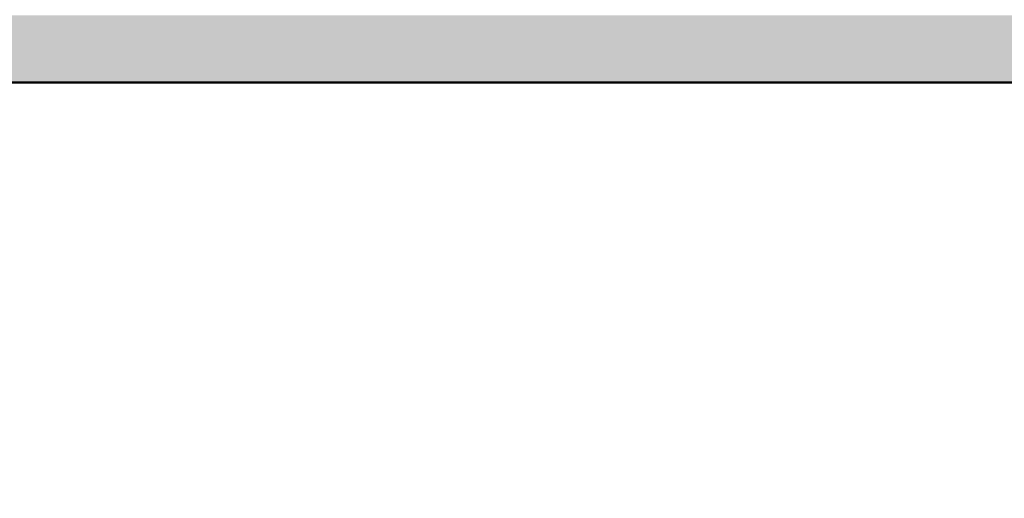
# Model space of a CAD drawing. Units: inches. Extents: x -7 to 1228, y -146 to 1091.
# Tile 44 of 88: x 81 to 169, y 531 to 574. Entities that reach past the tile are written whole.
import ezdxf

# ---------------------------------------------------------------- set-up
doc = ezdxf.new("R2010")
doc.units = ezdxf.units.IN
doc.layers.add('A-WALL', color=7, linetype='Continuous', lineweight=50)
doc.layers.add('A-WALL-PATT', color=251, linetype='Continuous', lineweight=13)

msp = doc.modelspace()

# ---------------------------------------------------------------- hatches: boundary and pattern name
at = {"layer": 'A-WALL-PATT'}
h = msp.add_hatch(color=256, dxfattribs=at)
h.dxf.hatch_style = 1
h.paths.add_polyline_path([(69, 568), (60, 568), (60, 493), (63.289, 493), (69, 493)])
h.paths.add_polyline_path([(69, 662.405), (60, 662.405), (60, 586), (69, 586)], flags=17)
h.paths.add_polyline_path([(69, 723), (184, 723), (184, 734), (179, 734), (179, 728), (69, 728), (69, 741.623), (60, 741.623), (60, 698.405), (69, 698.405)], flags=17)
h.paths.add_polyline_path([(69, 782), (231, 782), (231, 728), (231, 723), (231, 586), (236, 586), (236, 787), (69, 787), (69, 800.126), (60, 800.126), (60, 765.623), (69, 765.623)])
h.paths.add_polyline_path([(184, 842), (189, 842), (189, 848), (173, 848), (173, 842), (179, 842), (179, 787), (184, 787)])
h.paths.add_polyline_path([(118.22, 69), (69, 69), (69, 60), (118.22, 60)])
h.paths.add_polyline_path([(227, 69), (154.22, 69), (154.22, 60), (227, 60)])
h.paths.add_polyline_path([(236, 60), (232.711, 60), (227, 60), (227, 36), (236, 36)])
h.paths.add_polyline_path([(389, 60), (380, 60), (380, 36), (389, 36)])
h.paths.add_polyline_path([(384, 181), (380, 181), (380, 115), (380, 78), (384, 78)])
h.paths.add_polyline_path([(380, 115), (334.547, 115), (334.547, 109), (380, 109)])
h.paths.add_polyline_path([(274.547, 115), (236, 115), (236, 201), (232.711, 201), (231, 201), (231, 78), (236, 78), (236, 109), (274.547, 109)])
h.paths.add_polyline_path([(69, 123), (60, 123), (60, 78), (69, 78)])
h.paths.add_polyline_path([(69, 201), (60, 201), (60, 159), (69, 159)])
h.paths.add_polyline_path([(143, 219), (69, 219), (69, 213), (143, 213)], flags=17)
h.paths.add_polyline_path([(189, 219), (184, 219), (184, 274), (231, 274), (231, 219), (236, 219), (236, 279), (184, 279), (184, 297), (179, 297), (179, 279), (69, 279), (69, 290.912), (60, 290.912), (60, 262.179), (69, 262.179), (69, 274), (179, 274), (179, 219), (173, 219), (173, 213), (189, 213)])
h.paths.add_polyline_path([(69, 238.179), (60, 238.179), (60, 219), (69, 219)], flags=17)
h.paths.add_polyline_path([(69, 333), (60, 333), (60, 314.912), (69, 314.912), (69, 316.965)])
h.paths.add_polyline_path([(190, 338), (184, 338), (69, 338), (69, 333), (179, 333), (179, 327), (184, 327), (184, 333.021), (190, 333.046)])
h.paths.add_polyline_path([(69, 386.806), (60, 386.806), (60, 351), (69, 351)])
h.paths.add_polyline_path([(69, 475), (60, 475), (60, 422.806), (69, 422.806)])
h.paths.add_polyline_path([(236, 475), (231, 475), (231, 351.238), (236, 351.238)])
h.paths.add_polyline_path([(384, 475), (380, 475), (380, 362), (384, 362)])
h.paths.add_polyline_path([(547, 307), (439, 307), (439, 356), (445, 356), (445, 362), (433, 362), (433, 307), (380, 307), (380, 244), (380, 241), (384, 241), (384, 301), (433, 301), (433, 277), (439, 277), (439, 301), (547, 301)])
h.paths.add_polyline_path([(547, 241), (439, 241), (439, 247), (433, 247), (433, 235), (547, 235)])
h.paths.add_polyline_path([(450, 69), (440.286, 69), (424.889, 69), (389, 69), (389, 60), (450, 60)])
h.paths.add_polyline_path([(547, 69), (486, 69), (486, 60), (547, 60)])
h.paths.add_polyline_path([(556, 148.268), (547, 148.268), (547, 78), (556, 78)])
h.paths.add_polyline_path([(556, 223), (547, 223), (547, 195), (547, 184.268), (556, 184.268)])
h.paths.add_polyline_path([(556, 311.192), (547, 311.192), (547, 273.075), (556, 273.075)])
h.paths.add_polyline_path([(556, 344), (552.711, 344), (547, 344), (547, 335.192), (556, 335.192)])
h.paths.add_polyline_path([(556, 249.075), (547, 249.075), (547, 241), (556, 241)])
h.paths.add_polyline_path([(547, 362), (475, 362), (475, 356), (547, 356)], flags=0)
h.paths.add_polyline_path([(556, 399.621), (547, 399.621), (547, 362), (556, 362)])
h.paths.add_polyline_path([(556, 475), (547, 475), (547, 435.621), (556, 435.621)])
h.paths.add_polyline_path([(547, 493), (389, 493), (389, 487), (547, 487)])
h.paths.add_polyline_path([(380, 493), (278, 493), (278, 487), (380, 487)])
h.paths.add_polyline_path([(227, 493), (69, 493), (69, 487), (227, 487)])
h.paths.add_polyline_path([(643, 122.445), (634, 122.445), (634, 78), (643, 78)])
h.paths.add_polyline_path([(702.5, 69), (692.786, 69), (677.389, 69), (643, 69), (643, 60), (702.5, 60)])
h.paths.add_polyline_path([(798, 69), (738.5, 69), (738.5, 60), (798, 60)])
h.paths.add_polyline_path([(807, 60), (803.711, 60), (798, 60), (798, 36), (807, 36)])
h.paths.add_polyline_path([(807, 109), (846.751, 109), (846.751, 115), (807, 115), (807, 159), (802, 159), (802, 78), (807, 78)])
h.paths.add_polyline_path([(807, 201), (802, 201), (802, 195), (807, 195)])
h.paths.add_polyline_path([(643, 201), (634, 201), (634, 158.445), (643, 158.445)])
h.paths.add_polyline_path([(756, 225), (751, 225), (751, 219), (643, 219), (643, 213), (756, 213)])
h.paths.add_polyline_path([(643, 240.848), (634, 240.848), (634, 219), (643, 219)])
h.paths.add_polyline_path([(643, 274), (643, 288.629), (634, 288.629), (634, 264.848), (643, 264.848)])
h.paths.add_polyline_path([(802, 279), (756, 279), (756, 297), (751, 297), (751, 279), (643, 279), (643, 274), (751, 274), (751, 255), (756, 255), (756, 274), (802, 274)])
h.paths.add_polyline_path([(807, 333), (803.711, 333), (802, 333), (802, 279), (802, 274), (802, 219), (807, 219)])
h.paths.add_polyline_path([(956, 182), (951, 182), (951, 115), (906.751, 115), (906.751, 109), (951, 109), (951, 78), (956, 78)])
h.paths.add_polyline_path([(960, 60), (951, 60), (951, 36), (960, 36)])
h.paths.add_polyline_path([(1021, 69), (1005.781, 69), (960, 69), (960, 60), (1021, 60)])
h.paths.add_polyline_path([(956, 224), (951, 224), (951, 218), (956, 218)])
h.paths.add_polyline_path([(956, 302), (1004, 302), (1004, 278), (1010, 278), (1010, 302), (1118, 302), (1118, 290.809), (1127, 290.809), (1127, 326.968), (1118, 326.968), (1118, 320.966), (1118, 307), (1010, 307), (1010, 356), (1016, 356), (1016, 362), (1004, 362), (1004, 307), (951, 307), (951, 244), (951, 242), (954.289, 242), (956, 242)])
h.paths.add_polyline_path([(643, 333), (634, 333), (634, 312.629), (643, 312.629), (643, 316.965)])
h.paths.add_polyline_path([(756, 338), (643, 338), (643, 333), (751, 333), (751, 327), (756, 327)])
h.paths.add_polyline_path([(643, 388), (634, 388), (634, 351), (643, 351)])
h.paths.add_polyline_path([(807, 357), (802, 357), (802, 351), (807, 351)])
h.paths.add_polyline_path([(807, 475), (802, 475), (802, 393), (807, 393)])
h.paths.add_polyline_path([(643, 475), (634, 475), (634, 424), (643, 424)])
h.paths.add_polyline_path([(798, 493), (643, 493), (643, 487), (798, 487)])
h.paths.add_polyline_path([(634, 493), (556, 493), (556, 487), (634, 487)])
h.paths.add_polyline_path([(813, 493), (807, 493), (807, 487), (813, 487)])
h.paths.add_polyline_path([(951, 493), (849, 493), (849, 487), (951, 487)])
h.paths.add_polyline_path([(956, 484), (951, 484), (951, 374), (956, 374)])
h.paths.add_polyline_path([(1109, 493), (969, 493), (969, 487), (1109, 487)])
h.paths.add_polyline_path([(1127, 484), (1118, 484), (1118, 450.641), (1127, 450.641)])
h.paths.add_polyline_path([(1127, 414.641), (1118, 414.641), (1118, 365), (1127, 365)])
h.paths.add_polyline_path([(1109, 362), (1046, 362), (1046, 356), (1109, 356)], flags=17)
h.paths.add_polyline_path([(1127, 356), (1123.454, 356), (1118, 356), (1118, 350.968), (1127, 350.968)], flags=0)
h.paths.add_polyline_path([(1127, 266.809), (1118, 266.809), (1118, 262.361), (1118, 242), (1127, 242)], flags=17)
h.paths.add_polyline_path([(1118, 242), (1010, 242), (1010, 248), (1004, 248), (1004, 237), (1118, 237)])
h.paths.add_polyline_path([(1127, 224), (1118, 224), (1118, 170), (1127, 170)])
h.paths.add_polyline_path([(1127, 134), (1118, 134), (1118, 78), (1127, 78)])
h.paths.add_polyline_path([(1118, 69), (1057, 69), (1057, 60), (1118, 60)])
h.paths.add_polyline_path([(227, 571.546), (227, 574), (69, 574), (69, 568), (227, 568)])
h.paths.add_polyline_path([(380, 571.546), (380, 574), (278, 574), (278, 568), (380, 568)])
h.paths.add_polyline_path([(242, 574), (236, 574), (236, 568), (242, 568)])
h.paths.add_polyline_path([(547, 571.546), (547, 574), (389, 574), (389, 568), (547, 568)])
h.paths.add_polyline_path([(384, 733), (380, 733), (380, 586), (384, 586)])
h.paths.add_polyline_path([(556, 646), (634, 646), (634, 655), (547, 655), (547, 586), (556, 586)])
h.paths.add_polyline_path([(634, 574), (556, 574), (556, 568), (634, 568)])
h.paths.add_polyline_path([(643, 655), (634, 655), (634, 586), (643, 586)])
h.paths.add_polyline_path([(798, 574), (643, 574), (643, 568), (798, 568)])
h.paths.add_polyline_path([(643, 663.854), (634, 663.854), (634, 655), (643, 655)])
h.paths.add_polyline_path([(556, 676.967), (547, 676.967), (547, 655), (556, 655)])
h.paths.add_polyline_path([(556, 733), (547, 733), (547, 712.967), (556, 712.967)])
h.paths.add_polyline_path([(643, 710), (634, 710), (634, 699.854), (643, 699.854)])
h.paths.add_polyline_path([(807, 668), (802, 668), (802, 586), (807, 586)])
h.paths.add_polyline_path([(951, 574), (849, 574), (849, 568), (951, 568)])
h.paths.add_polyline_path([(956, 691), (951, 691), (951, 577), (956, 577)])
h.paths.add_polyline_path([(1109, 574), (969, 574), (969, 568), (1109, 568)])
h.paths.add_polyline_path([(1127, 643.403), (1118, 643.403), (1118, 577), (1127, 577)])
h.paths.add_polyline_path([(1127, 568), (1123.454, 568), (1118, 568), (1118, 493), (1127, 493)])
h.paths.add_polyline_path([(1127, 733), (1118, 733), (1118, 679.403), (1127, 679.403)])
h.paths.add_polyline_path([(1127, 777.348), (1118, 777.348), (1118, 770.035), (1118, 751), (1127, 751)], flags=17)
h.paths.add_polyline_path([(1118, 751), (1010, 751), (1010, 757), (1004, 757), (1004, 745), (1118, 745)])
h.paths.add_polyline_path([(956, 811), (1004, 811), (1004, 787), (1010, 787), (1010, 811), (1017.874, 811), (1017.874, 811.627, -0.414214), (1018.247, 812), (1031.978, 812, -0.414214), (1032.351, 811.627), (1032.351, 811), (1118, 811), (1118, 801.348), (1127, 801.348), (1127, 834.685), (1118, 834.685), (1118, 830.238), (1118, 817), (1010, 817), (1010, 866), (1016, 866), (1016, 872), (1004, 872), (1004, 817), (956, 817), (956, 866), (951, 866), (951, 751), (954.289, 751), (956, 751)])
h.paths.add_polyline_path([(1118, 872), (1046, 872), (1046, 866), (1118, 866)], flags=17)
h.paths.add_polyline_path([(1127, 924.711), (1118, 924.711), (1118, 884), (1127, 884)])
h.paths.add_polyline_path([(1127, 866), (1123.711, 866), (1118, 866), (1118, 858.685), (1127, 858.685)], flags=17)
h.paths.add_polyline_path([(956, 983), (951, 983), (951, 952), (807, 952), (807, 983), (802, 983), (802, 902), (807, 902), (807, 946), (951, 946), (951, 884), (956, 884)])
h.paths.add_polyline_path([(807, 842), (802, 842), (802, 787), (756, 787), (756, 806), (751, 806), (751, 787), (643, 787), (643, 782), (751, 782), (751, 764), (756, 764), (756, 782), (802, 782), (802, 728), (807, 728)])
h.paths.add_polyline_path([(756, 848), (643, 848), (643, 842), (751, 842), (751, 836), (756, 836)])
h.paths.add_polyline_path([(756, 734), (751, 734), (751, 728), (643, 728), (643, 723), (756, 723)])
h.paths.add_polyline_path([(643, 749.791), (634, 749.791), (634, 728), (637.289, 728), (643, 728)])
h.paths.add_polyline_path([(643, 805.405), (634, 805.405), (634, 773.791), (643, 773.791)])
h.paths.add_polyline_path([(643, 896.663), (634, 896.663), (634, 860), (637.289, 860), (643, 860)])
h.paths.add_polyline_path([(643, 842), (634, 842), (634, 829.405), (643, 829.405)])
h.paths.add_polyline_path([(643, 983), (634, 983), (634, 932.663), (643, 932.663)])
h.paths.add_polyline_path([(1127, 983), (1118, 983), (1118, 960.711), (1127, 960.711)])
h.paths.add_polyline_path([(1118, 1001), (1077.525, 1001), (1077.525, 992), (1118, 992)])
h.paths.add_polyline_path([(1041.525, 1001), (960, 1001), (960, 992), (1041.525, 992)])
h.paths.add_polyline_path([(960, 1025), (951, 1025), (951, 1001), (954.289, 1001), (960, 1001)])
h.paths.add_polyline_path([(807, 1025), (798, 1025), (798, 1001), (807, 1001)])
h.paths.add_polyline_path([(798, 1001), (738.5, 1001), (738.5, 992), (798, 992)])
h.paths.add_polyline_path([(702.5, 1001), (643, 1001), (643, 992), (702.5, 992)])
h.paths.add_polyline_path([(547, 1001), (499.113, 1001), (499.113, 992), (547, 992)])
h.paths.add_polyline_path([(463.113, 1001), (389, 1001), (389, 992), (463.113, 992)])
h.paths.add_polyline_path([(389, 1025), (380, 1025), (380, 1022), (380, 1001), (383.289, 1001), (389, 1001)])
h.paths.add_polyline_path([(236, 1025), (227, 1025), (227, 1001), (236, 1001)])
h.paths.add_polyline_path([(236, 983), (231, 983), (231, 860), (236, 860)])
h.paths.add_polyline_path([(274.547, 952), (236, 952), (236, 946), (274.547, 946)])
h.paths.add_polyline_path([(380, 952), (334.547, 952), (334.547, 946), (380, 946)])
h.paths.add_polyline_path([(384, 983), (380, 983), (380, 884), (383.289, 884), (384, 884)])
h.paths.add_polyline_path([(227, 1001), (155.012, 1001), (155.012, 992), (162.875, 992), (227, 992)])
h.paths.add_polyline_path([(119.012, 1001), (69, 1001), (69, 992), (119.012, 992)])
h.paths.add_polyline_path([(69, 983), (60, 983), (60, 922.987), (69, 922.987)])
h.paths.add_polyline_path([(69, 886.987), (60, 886.987), (60, 860), (63.289, 860), (69, 860)])
h.paths.add_polyline_path([(143, 848), (69, 848), (69, 842), (143, 842)])

# ---------------------------------------------------------------- linework, layer by layer
at = {"layer": 'A-WALL'}
msp.add_line((231, 568), (60, 568), dxfattribs=at)

doc.saveas('drawing.dxf')
